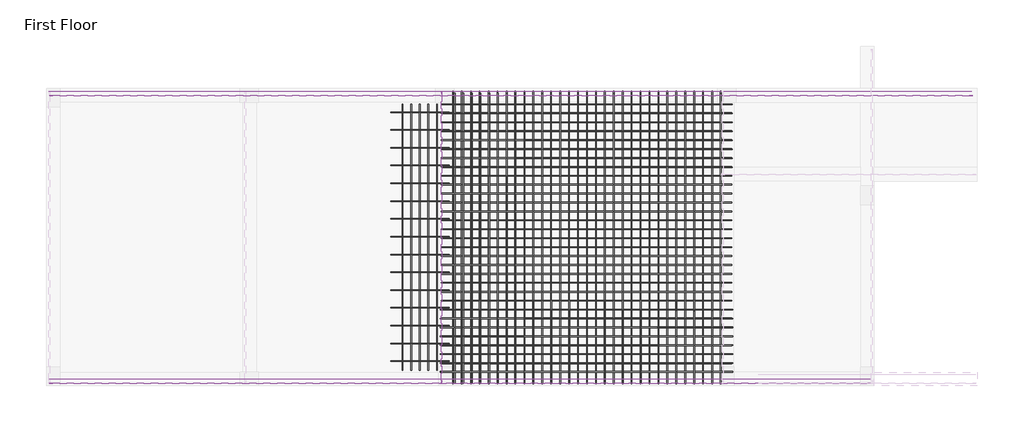
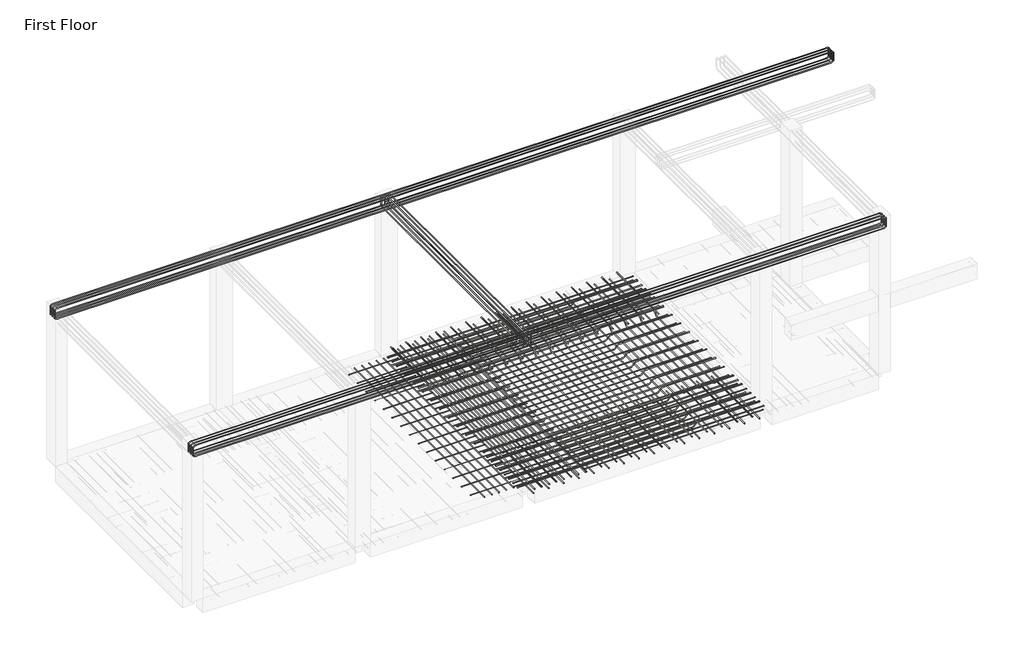
# One storey, part 3 of 4: 18 reinforcing bars.
"""IFC4 building model written with IfcOpenShell, lengths in millimetres."""

from ifc_helpers import new_model, si_unit, point, frame, origin, place, context, project, spatial, polyline, circle_curve, trimmed, segment, composite_curve, source, transform, mapped, element, save
from ifc_brep_helpers import swept_disk

model = new_model("IFC4")

# Units and contexts
model_context = context("Model", 3, world=origin())
ifc_project = project(units=[si_unit("LENGTHUNIT", "METRE", prefix="MILLI")], contexts=[model_context])

# Site, building, storey
site = spatial("IfcSite", under=ifc_project)
building = spatial("IfcBuilding", under=site)
storey = spatial("IfcBuildingStorey", under=building, Name="First Floor", Elevation=3200.4)

# Reinforcing bars
placement = place(None, origin())
reinforcing_bar_shape = source(origin(), model_context, "Body", "SolidModel", [
    swept_disk(composite_curve([segment(polyline([(-2909.6112474, 5017.2334631, 6163.6994949), (-2909.6112474, 5017.2334631, 6311.6994949)]), True, "CONTINUOUS"), segment(trimmed(circle_curve(frame((-2909.6112474, 4971.2334631, 6311.6994949), z_axis=(1.0, 0.0, 0.0), x_axis=(0.0, 46.0, 0.0)), 46.0), [point((-2909.6112474, 5017.2334631, 6311.6994949))], [point((-2909.6112474, 4971.2334631, 6357.6994949))], True, "CARTESIAN"), True, "CONTINUOUS"), segment(polyline([(-2909.6112474, 4971.2334631, 6357.6994949), (-2909.6112474, 278.4334631, 6357.6994949)]), True, "CONTINUOUS"), segment(trimmed(circle_curve(frame((-2909.6112474, 278.4334631, 6311.6994949), z_axis=(1.0, 0.0, 0.0), x_axis=(0.0, 0.0, 46.0)), 46.0), [point((-2909.6112474, 278.4334631, 6357.6994949))], [point((-2909.6112474, 232.4334631, 6311.6994949))], True, "CARTESIAN"), True, "CONTINUOUS"), segment(polyline([(-2909.6112474, 232.4334631, 6311.6994949), (-2909.6112474, 232.4334631, 6163.6994949)]), True, "CONTINUOUS")], self_intersect=False), 6.0),
])
element("IfcReinforcingBar", 1, at=placement, inside=storey, context=model_context, shape_type="MappedRepresentation", body=[
    mapped(reinforcing_bar_shape, transform((0.0, 0.0, 0.0), x_axis=(1.0, 0.0, 0.0), y_axis=(0.0, 1.0, 0.0), z_axis=(0.0, 0.0, 1.0))),
    mapped(reinforcing_bar_shape, transform((71.1994949, 0.0, 0.0), x_axis=(1.0, 0.0, 0.0), y_axis=(0.0, 1.0, 0.0), z_axis=(0.0, 0.0, 1.0))),
    mapped(reinforcing_bar_shape, transform((142.3989899, 0.0, 0.0), x_axis=(1.0, 0.0, 0.0), y_axis=(0.0, 1.0, 0.0), z_axis=(0.0, 0.0, 1.0))),
])
reinforcing_bar_2_shape = source(origin(), model_context, "Body", "SolidModel", [
    swept_disk(composite_curve([segment(polyline([(-2909.6112474, 5017.2334631, 6333.1005051), (-2909.6112474, 5017.2334631, 6185.1005051)]), True, "CONTINUOUS"), segment(trimmed(circle_curve(frame((-2909.6112474, 4971.2334631, 6185.1005051), z_axis=(-1.0, 0.0, 0.0), x_axis=(0.0, 46.0, 0.0)), 46.0), [point((-2909.6112474, 5017.2334631, 6185.1005051))], [point((-2909.6112474, 4971.2334631, 6139.1005051))], True, "CARTESIAN"), True, "CONTINUOUS"), segment(polyline([(-2909.6112474, 4971.2334631, 6139.1005051), (-2909.6112474, 278.4334631, 6139.1005051)]), True, "CONTINUOUS"), segment(trimmed(circle_curve(frame((-2909.6112474, 278.4334631, 6185.1005051), z_axis=(-1.0, 0.0, 0.0), x_axis=(0.0, 0.0, -46.0)), 46.0), [point((-2909.6112474, 278.4334631, 6139.1005051))], [point((-2909.6112474, 232.4334631, 6185.1005051))], True, "CARTESIAN"), True, "CONTINUOUS"), segment(polyline([(-2909.6112474, 232.4334631, 6185.1005051), (-2909.6112474, 232.4334631, 6333.1005051)]), True, "CONTINUOUS")], self_intersect=False), 6.0),
])
element("IfcReinforcingBar", 2, at=placement, inside=storey, context=model_context, shape_type="MappedRepresentation", body=[
    mapped(reinforcing_bar_2_shape, transform((0.0, 0.0, 0.0), x_axis=(1.0, 0.0, 0.0), y_axis=(0.0, 1.0, 0.0), z_axis=(0.0, 0.0, 1.0))),
    mapped(reinforcing_bar_2_shape, transform((71.1994949, 0.0, 0.0), x_axis=(1.0, 0.0, 0.0), y_axis=(0.0, 1.0, 0.0), z_axis=(0.0, 0.0, 1.0))),
    mapped(reinforcing_bar_2_shape, transform((142.3989899, 0.0, 0.0), x_axis=(1.0, 0.0, 0.0), y_axis=(0.0, 1.0, 0.0), z_axis=(0.0, 0.0, 1.0))),
])
reinforcing_bar_3_shape = source(origin(), model_context, "Body", "SolidModel", [
    swept_disk(composite_curve([segment(polyline([(-9325.7296265, 229.5339681, 6163.6994949), (-9325.7296265, 229.5339681, 6311.6994949)]), True, "CONTINUOUS"), segment(trimmed(circle_curve(frame((-9279.7296265, 229.5339681, 6311.6994949), z_axis=(0.0, 1.0, 0.0), x_axis=(-46.0, 0.0, 0.0)), 46.0), [point((-9325.7296265, 229.5339681, 6311.6994949))], [point((-9279.7296265, 229.5339681, 6357.6994949))], True, "CARTESIAN"), True, "CONTINUOUS"), segment(polyline([(-9279.7296265, 229.5339681, 6357.6994949), (4070.8650323, 229.5339681, 6357.6994949)]), True, "CONTINUOUS"), segment(trimmed(circle_curve(frame((4070.8650323, 229.5339681, 6311.6994949), z_axis=(0.0, 1.0, 0.0), x_axis=(0.0, 0.0, 46.0)), 46.0), [point((4070.8650323, 229.5339681, 6357.6994949))], [point((4116.8650323, 229.5339681, 6311.6994949))], True, "CARTESIAN"), True, "CONTINUOUS"), segment(polyline([(4116.8650323, 229.5339681, 6311.6994949), (4116.8650323, 229.5339681, 6163.6994949)]), True, "CONTINUOUS")], self_intersect=False), 6.0),
])
element("IfcReinforcingBar", 3, at=placement, inside=storey, context=model_context, shape_type="MappedRepresentation", body=[
    mapped(reinforcing_bar_3_shape, transform((0.0, 0.0, 0.0), x_axis=(1.0, 0.0, 0.0), y_axis=(0.0, 1.0, 0.0), z_axis=(0.0, 0.0, 1.0))),
    mapped(reinforcing_bar_3_shape, transform((0.0, 71.1994949, 0.0), x_axis=(1.0, 0.0, 0.0), y_axis=(0.0, 1.0, 0.0), z_axis=(0.0, 0.0, 1.0))),
    mapped(reinforcing_bar_3_shape, transform((0.0, 142.3989899, 0.0), x_axis=(1.0, 0.0, 0.0), y_axis=(0.0, 1.0, 0.0), z_axis=(0.0, 0.0, 1.0))),
])
reinforcing_bar_4_shape = source(origin(), model_context, "Body", "SolidModel", [
    swept_disk(composite_curve([segment(polyline([(-9326.1203644, 229.5339681, 6333.1005051), (-9326.1203644, 229.5339681, 6185.1005051)]), True, "CONTINUOUS"), segment(trimmed(circle_curve(frame((-9280.1203644, 229.5339681, 6185.1005051), z_axis=(0.0, -1.0, 0.0), x_axis=(-46.0, 0.0, 0.0)), 46.0), [point((-9326.1203644, 229.5339681, 6185.1005051))], [point((-9280.1203644, 229.5339681, 6139.1005051))], True, "CARTESIAN"), True, "CONTINUOUS"), segment(polyline([(-9280.1203644, 229.5339681, 6139.1005051), (4076.5679264, 229.5339681, 6139.1005051)]), True, "CONTINUOUS"), segment(trimmed(circle_curve(frame((4076.5679264, 229.5339681, 6185.1005051), z_axis=(0.0, -1.0, 0.0), x_axis=(0.0, 0.0, -46.0)), 46.0), [point((4076.5679264, 229.5339681, 6139.1005051))], [point((4122.5679264, 229.5339681, 6185.1005051))], True, "CARTESIAN"), True, "CONTINUOUS"), segment(polyline([(4122.5679264, 229.5339681, 6185.1005051), (4122.5679264, 229.5339681, 6333.1005051)]), True, "CONTINUOUS")], self_intersect=False), 6.0),
])
element("IfcReinforcingBar", 4, at=placement, inside=storey, context=model_context, shape_type="MappedRepresentation", body=[
    mapped(reinforcing_bar_4_shape, transform((0.0, 0.0, 0.0), x_axis=(1.0, 0.0, 0.0), y_axis=(0.0, 1.0, 0.0), z_axis=(0.0, 0.0, 1.0))),
    mapped(reinforcing_bar_4_shape, transform((0.0, 71.1994949, 0.0), x_axis=(1.0, 0.0, 0.0), y_axis=(0.0, 1.0, 0.0), z_axis=(0.0, 0.0, 1.0))),
    mapped(reinforcing_bar_4_shape, transform((0.0, 142.3989899, 0.0), x_axis=(1.0, 0.0, 0.0), y_axis=(0.0, 1.0, 0.0), z_axis=(0.0, 0.0, 1.0))),
])
reinforcing_bar_5_shape = source(origin(), model_context, "Body", "SolidModel", [
    swept_disk(composite_curve([segment(polyline([(-9325.7296265, 4879.1314555, 6162.3020076), (-9325.7296265, 4879.1314555, 6310.3020076)]), True, "CONTINUOUS"), segment(trimmed(circle_curve(frame((-9279.7296265, 4879.1314555, 6310.3020076), z_axis=(0.0, 1.0, 0.0), x_axis=(-46.0, 0.0, 0.0)), 46.0), [point((-9325.7296265, 4879.1314555, 6310.3020076))], [point((-9279.7296265, 4879.1314555, 6356.3020076))], True, "CARTESIAN"), True, "CONTINUOUS"), segment(polyline([(-9279.7296265, 4879.1314555, 6356.3020076), (5739.4882476, 4879.1314555, 6356.3020076)]), True, "CONTINUOUS"), segment(trimmed(circle_curve(frame((5739.4882476, 4879.1314555, 6310.3020076), z_axis=(0.0, 1.0, 0.0), x_axis=(0.0, 0.0, 46.0)), 46.0), [point((5739.4882476, 4879.1314555, 6356.3020076))], [point((5785.4882476, 4879.1314555, 6310.3020076))], True, "CARTESIAN"), True, "CONTINUOUS"), segment(polyline([(5785.4882476, 4879.1314555, 6310.3020076), (5785.4882476, 4879.1314555, 6162.3020076)]), True, "CONTINUOUS")], self_intersect=False), 6.0),
])
element("IfcReinforcingBar", 5, at=placement, inside=storey, context=model_context, shape_type="MappedRepresentation", body=[
    mapped(reinforcing_bar_5_shape, transform((0.0, 0.0, 0.0), x_axis=(1.0, 0.0, 0.0), y_axis=(0.0, 1.0, 0.0), z_axis=(0.0, 0.0, 1.0))),
    mapped(reinforcing_bar_5_shape, transform((0.0, 69.8020076, 0.0), x_axis=(1.0, 0.0, 0.0), y_axis=(0.0, 1.0, 0.0), z_axis=(0.0, 0.0, 1.0))),
    mapped(reinforcing_bar_5_shape, transform((0.0, 139.6040151, 0.0), x_axis=(1.0, 0.0, 0.0), y_axis=(0.0, 1.0, 0.0), z_axis=(0.0, 0.0, 1.0))),
])
reinforcing_bar_6_shape = source(origin(), model_context, "Body", "SolidModel", [
    swept_disk(composite_curve([segment(polyline([(-9326.1203644, 4879.1314555, 6334.8479924), (-9326.1203644, 4879.1314555, 6186.8479924)]), True, "CONTINUOUS"), segment(trimmed(circle_curve(frame((-9280.1203644, 4879.1314555, 6186.8479924), z_axis=(0.0, -1.0, 0.0), x_axis=(-46.0, 0.0, 0.0)), 46.0), [point((-9326.1203644, 4879.1314555, 6186.8479924))], [point((-9280.1203644, 4879.1314555, 6140.8479924))], True, "CARTESIAN"), True, "CONTINUOUS"), segment(polyline([(-9280.1203644, 4879.1314555, 6140.8479924), (5727.8951301, 4879.1314555, 6140.8479924)]), True, "CONTINUOUS"), segment(trimmed(circle_curve(frame((5727.8951301, 4879.1314555, 6186.8479924), z_axis=(0.0, -1.0, 0.0), x_axis=(0.0, 0.0, -46.0)), 46.0), [point((5727.8951301, 4879.1314555, 6140.8479924))], [point((5773.8951301, 4879.1314555, 6186.8479924))], True, "CARTESIAN"), True, "CONTINUOUS"), segment(polyline([(5773.8951301, 4879.1314555, 6186.8479924), (5773.8951301, 4879.1314555, 6334.8479924)]), True, "CONTINUOUS")], self_intersect=False), 6.0),
])
element("IfcReinforcingBar", 6, at=placement, inside=storey, context=model_context, shape_type="MappedRepresentation", body=[
    mapped(reinforcing_bar_6_shape, transform((0.0, 0.0, 0.0), x_axis=(1.0, 0.0, 0.0), y_axis=(0.0, 1.0, 0.0), z_axis=(0.0, 0.0, 1.0))),
    mapped(reinforcing_bar_6_shape, transform((0.0, 69.8020076, 0.0), x_axis=(1.0, 0.0, 0.0), y_axis=(0.0, 1.0, 0.0), z_axis=(0.0, 0.0, 1.0))),
    mapped(reinforcing_bar_6_shape, transform((0.0, 139.6040151, 0.0), x_axis=(1.0, 0.0, 0.0), y_axis=(0.0, 1.0, 0.0), z_axis=(0.0, 0.0, 1.0))),
])
reinforcing_bar_7_shape = source(origin(), model_context, "Body", "SolidModel", [
    swept_disk(composite_curve([segment(polyline([(-3546.4250876, 4809.6334631, 3159.1006995), (-3546.4250876, 440.0334631, 3159.1006995)]), True, "CONTINUOUS")], self_intersect=False), 6.0),
])
element("IfcReinforcingBar", 7, at=placement, inside=storey, context=model_context, shape_type="MappedRepresentation", body=[
    mapped(reinforcing_bar_7_shape, transform((0.0, 0.0, 0.0), x_axis=(1.0, 0.0, 0.0), y_axis=(0.0, 1.0, 0.0), z_axis=(0.0, 0.0, 1.0))),
    mapped(reinforcing_bar_7_shape, transform((140.6783338, 0.0, 0.0), x_axis=(1.0, 0.0, 0.0), y_axis=(0.0, 1.0, 0.0), z_axis=(0.0, 0.0, 1.0))),
    mapped(reinforcing_bar_7_shape, transform((281.3566676, 0.0, 0.0), x_axis=(1.0, 0.0, 0.0), y_axis=(0.0, 1.0, 0.0), z_axis=(0.0, 0.0, 1.0))),
    mapped(reinforcing_bar_7_shape, transform((422.0350014, 0.0, 0.0), x_axis=(1.0, 0.0, 0.0), y_axis=(0.0, 1.0, 0.0), z_axis=(0.0, 0.0, 1.0))),
    mapped(reinforcing_bar_7_shape, transform((562.7133352, 0.0, 0.0), x_axis=(1.0, 0.0, 0.0), y_axis=(0.0, 1.0, 0.0), z_axis=(0.0, 0.0, 1.0))),
])
reinforcing_bar_8_shape = source(origin(), model_context, "Body", "SolidModel", [
    swept_disk(composite_curve([segment(polyline([(-2778.2123639, 4678.4115375, 3171.4), (-3737.2865297, 4678.4115375, 3171.4)]), True, "CONTINUOUS")], self_intersect=False), 4.0),
])
element("IfcReinforcingBar", 8, at=placement, inside=storey, context=model_context, shape_type="MappedRepresentation", body=[
    mapped(reinforcing_bar_8_shape, transform((0.0, 0.0, 0.0), x_axis=(1.0, 0.0, 0.0), y_axis=(0.0, 1.0, 0.0), z_axis=(0.0, 0.0, 1.0))),
    mapped(reinforcing_bar_8_shape, transform((0.0, -291.8025106, 0.0), x_axis=(1.0, 0.0, 0.0), y_axis=(0.0, 1.0, 0.0), z_axis=(0.0, 0.0, 1.0))),
    mapped(reinforcing_bar_8_shape, transform((0.0, -583.6050212, 0.0), x_axis=(1.0, 0.0, 0.0), y_axis=(0.0, 1.0, 0.0), z_axis=(0.0, 0.0, 1.0))),
    mapped(reinforcing_bar_8_shape, transform((0.0, -875.4075319, 0.0), x_axis=(1.0, 0.0, 0.0), y_axis=(0.0, 1.0, 0.0), z_axis=(0.0, 0.0, 1.0))),
    mapped(reinforcing_bar_8_shape, transform((0.0, -1167.2100425, 0.0), x_axis=(1.0, 0.0, 0.0), y_axis=(0.0, 1.0, 0.0), z_axis=(0.0, 0.0, 1.0))),
    mapped(reinforcing_bar_8_shape, transform((0.0, -1459.0125531, 0.0), x_axis=(1.0, 0.0, 0.0), y_axis=(0.0, 1.0, 0.0), z_axis=(0.0, 0.0, 1.0))),
    mapped(reinforcing_bar_8_shape, transform((0.0, -1750.8150637, 0.0), x_axis=(1.0, 0.0, 0.0), y_axis=(0.0, 1.0, 0.0), z_axis=(0.0, 0.0, 1.0))),
    mapped(reinforcing_bar_8_shape, transform((0.0, -2042.6175743, 0.0), x_axis=(1.0, 0.0, 0.0), y_axis=(0.0, 1.0, 0.0), z_axis=(0.0, 0.0, 1.0))),
    mapped(reinforcing_bar_8_shape, transform((0.0, -2334.420085, 0.0), x_axis=(1.0, 0.0, 0.0), y_axis=(0.0, 1.0, 0.0), z_axis=(0.0, 0.0, 1.0))),
    mapped(reinforcing_bar_8_shape, transform((0.0, -2626.2225956, 0.0), x_axis=(1.0, 0.0, 0.0), y_axis=(0.0, 1.0, 0.0), z_axis=(0.0, 0.0, 1.0))),
    mapped(reinforcing_bar_8_shape, transform((0.0, -2918.0251062, 0.0), x_axis=(1.0, 0.0, 0.0), y_axis=(0.0, 1.0, 0.0), z_axis=(0.0, 0.0, 1.0))),
    mapped(reinforcing_bar_8_shape, transform((0.0, -3209.8276168, 0.0), x_axis=(1.0, 0.0, 0.0), y_axis=(0.0, 1.0, 0.0), z_axis=(0.0, 0.0, 1.0))),
    mapped(reinforcing_bar_8_shape, transform((0.0, -3501.6301274, 0.0), x_axis=(1.0, 0.0, 0.0), y_axis=(0.0, 1.0, 0.0), z_axis=(0.0, 0.0, 1.0))),
    mapped(reinforcing_bar_8_shape, transform((0.0, -3793.4326381, 0.0), x_axis=(1.0, 0.0, 0.0), y_axis=(0.0, 1.0, 0.0), z_axis=(0.0, 0.0, 1.0))),
    mapped(reinforcing_bar_8_shape, transform((0.0, -4085.2351487, 0.0), x_axis=(1.0, 0.0, 0.0), y_axis=(0.0, 1.0, 0.0), z_axis=(0.0, 0.0, 1.0))),
])
reinforcing_bar_9_shape = source(origin(), model_context, "Body", "SolidModel", [
    swept_disk(composite_curve([segment(polyline([(-1702.6950858, 4992.3164819, 3154.1006995), (-1702.6950858, 234.3272052, 3154.1006995)]), True, "CONTINUOUS")], self_intersect=False), 6.0),
])
element("IfcReinforcingBar", 9, at=placement, inside=storey, context=model_context, shape_type="MappedRepresentation", body=[
    mapped(reinforcing_bar_9_shape, transform((0.0, 0.0, 0.0), x_axis=(1.0, 0.0, 0.0), y_axis=(0.0, 1.0, 0.0), z_axis=(0.0, 0.0, 1.0))),
    mapped(reinforcing_bar_9_shape, transform((-141.4880952, 0.0, 0.0), x_axis=(1.0, 0.0, 0.0), y_axis=(0.0, 1.0, 0.0), z_axis=(0.0, 0.0, 1.0))),
    mapped(reinforcing_bar_9_shape, transform((-282.9761905, 0.0, 0.0), x_axis=(1.0, 0.0, 0.0), y_axis=(0.0, 1.0, 0.0), z_axis=(0.0, 0.0, 1.0))),
    mapped(reinforcing_bar_9_shape, transform((-424.4642857, 0.0, 0.0), x_axis=(1.0, 0.0, 0.0), y_axis=(0.0, 1.0, 0.0), z_axis=(0.0, 0.0, 1.0))),
    mapped(reinforcing_bar_9_shape, transform((-565.952381, 0.0, 0.0), x_axis=(1.0, 0.0, 0.0), y_axis=(0.0, 1.0, 0.0), z_axis=(0.0, 0.0, 1.0))),
    mapped(reinforcing_bar_9_shape, transform((-707.4404762, 0.0, 0.0), x_axis=(1.0, 0.0, 0.0), y_axis=(0.0, 1.0, 0.0), z_axis=(0.0, 0.0, 1.0))),
    mapped(reinforcing_bar_9_shape, transform((-848.9285714, 0.0, 0.0), x_axis=(1.0, 0.0, 0.0), y_axis=(0.0, 1.0, 0.0), z_axis=(0.0, 0.0, 1.0))),
    mapped(reinforcing_bar_9_shape, transform((-990.4166667, 0.0, 0.0), x_axis=(1.0, 0.0, 0.0), y_axis=(0.0, 1.0, 0.0), z_axis=(0.0, 0.0, 1.0))),
])
reinforcing_bar_10_shape = source(origin(), model_context, "Body", "SolidModel", [
    swept_disk(composite_curve([segment(polyline([(-2905.905155, 4803.6334631, 3166.3687876), (-1727.9771661, 4803.6334631, 3166.3687876)]), True, "CONTINUOUS"), segment(trimmed(circle_curve(frame((-1727.9771661, 4803.6334631, 3120.3687876), z_axis=(0.0, 1.0, 0.0), x_axis=(0.0, 0.0, 46.0)), 46.0), [point((-1727.9771661, 4803.6334631, 3166.3687876))], [point((-1695.4502541, 4803.6334631, 3152.8956996))], True, "CARTESIAN"), True, "CONTINUOUS"), segment(polyline([(-1695.4502541, 4803.6334631, 3152.8956996), (-1634.9899166, 4803.6334631, 3092.4353621)]), True, "CONTINUOUS"), segment(trimmed(circle_curve(frame((-1602.4630047, 4803.6334631, 3124.962274), z_axis=(0.0, -1.0, 0.0), x_axis=(-32.52691189999996, 0.0, -32.52691189999996)), 46.0), [point((-1634.9899166, 4803.6334631, 3092.4353621))], [point((-1602.4630047, 4803.6334631, 3078.962274))], True, "CARTESIAN"), True, "CONTINUOUS"), segment(polyline([(-1602.4630047, 4803.6334631, 3078.962274), (1847.5013288, 4803.6334631, 3078.962274)]), True, "CONTINUOUS")], self_intersect=False), 6.0),
])
element("IfcReinforcingBar", 10, at=placement, inside=storey, context=model_context, shape_type="MappedRepresentation", body=[
    mapped(reinforcing_bar_10_shape, transform((0.0, 0.0, 0.0), x_axis=(1.0, 0.0, 0.0), y_axis=(0.0, 1.0, 0.0), z_axis=(0.0, 0.0, 1.0))),
    mapped(reinforcing_bar_10_shape, transform((0.0, -292.3066667, 0.0), x_axis=(1.0, 0.0, 0.0), y_axis=(0.0, 1.0, 0.0), z_axis=(0.0, 0.0, 1.0))),
    mapped(reinforcing_bar_10_shape, transform((0.0, -584.6133333, 0.0), x_axis=(1.0, 0.0, 0.0), y_axis=(0.0, 1.0, 0.0), z_axis=(0.0, 0.0, 1.0))),
    mapped(reinforcing_bar_10_shape, transform((0.0, -876.92, 0.0), x_axis=(1.0, 0.0, 0.0), y_axis=(0.0, 1.0, 0.0), z_axis=(0.0, 0.0, 1.0))),
    mapped(reinforcing_bar_10_shape, transform((0.0, -1169.2266667, 0.0), x_axis=(1.0, 0.0, 0.0), y_axis=(0.0, 1.0, 0.0), z_axis=(0.0, 0.0, 1.0))),
    mapped(reinforcing_bar_10_shape, transform((0.0, -1461.5333333, 0.0), x_axis=(1.0, 0.0, 0.0), y_axis=(0.0, 1.0, 0.0), z_axis=(0.0, 0.0, 1.0))),
    mapped(reinforcing_bar_10_shape, transform((0.0, -1753.84, 0.0), x_axis=(1.0, 0.0, 0.0), y_axis=(0.0, 1.0, 0.0), z_axis=(0.0, 0.0, 1.0))),
    mapped(reinforcing_bar_10_shape, transform((0.0, -2046.1466667, 0.0), x_axis=(1.0, 0.0, 0.0), y_axis=(0.0, 1.0, 0.0), z_axis=(0.0, 0.0, 1.0))),
    mapped(reinforcing_bar_10_shape, transform((0.0, -2338.4533333, 0.0), x_axis=(1.0, 0.0, 0.0), y_axis=(0.0, 1.0, 0.0), z_axis=(0.0, 0.0, 1.0))),
    mapped(reinforcing_bar_10_shape, transform((0.0, -2630.76, 0.0), x_axis=(1.0, 0.0, 0.0), y_axis=(0.0, 1.0, 0.0), z_axis=(0.0, 0.0, 1.0))),
    mapped(reinforcing_bar_10_shape, transform((0.0, -2923.0666667, 0.0), x_axis=(1.0, 0.0, 0.0), y_axis=(0.0, 1.0, 0.0), z_axis=(0.0, 0.0, 1.0))),
    mapped(reinforcing_bar_10_shape, transform((0.0, -3215.3733333, 0.0), x_axis=(1.0, 0.0, 0.0), y_axis=(0.0, 1.0, 0.0), z_axis=(0.0, 0.0, 1.0))),
    mapped(reinforcing_bar_10_shape, transform((0.0, -3507.68, 0.0), x_axis=(1.0, 0.0, 0.0), y_axis=(0.0, 1.0, 0.0), z_axis=(0.0, 0.0, 1.0))),
    mapped(reinforcing_bar_10_shape, transform((0.0, -3799.9866667, 0.0), x_axis=(1.0, 0.0, 0.0), y_axis=(0.0, 1.0, 0.0), z_axis=(0.0, 0.0, 1.0))),
    mapped(reinforcing_bar_10_shape, transform((0.0, -4092.2933333, 0.0), x_axis=(1.0, 0.0, 0.0), y_axis=(0.0, 1.0, 0.0), z_axis=(0.0, 0.0, 1.0))),
    mapped(reinforcing_bar_10_shape, transform((0.0, -4384.6, 0.0), x_axis=(1.0, 0.0, 0.0), y_axis=(0.0, 1.0, 0.0), z_axis=(0.0, 0.0, 1.0))),
])
reinforcing_bar_11_shape = source(origin(), model_context, "Body", "SolidModel", [
    swept_disk(composite_curve([segment(polyline([(-2911.6309684, 4803.6334631, 3163.8017937), (-1557.9199073, 4803.6334631, 3163.8017937)]), True, "CONTINUOUS")], self_intersect=False), 6.0),
])
element("IfcReinforcingBar", 11, at=placement, inside=storey, context=model_context, shape_type="MappedRepresentation", body=[
    mapped(reinforcing_bar_11_shape, transform((0.0, 0.0, 0.0), x_axis=(1.0, 0.0, 0.0), y_axis=(0.0, 1.0, 0.0), z_axis=(0.0, 0.0, 1.0))),
    mapped(reinforcing_bar_11_shape, transform((0.0, -292.3066667, 0.0), x_axis=(1.0, 0.0, 0.0), y_axis=(0.0, 1.0, 0.0), z_axis=(0.0, 0.0, 1.0))),
    mapped(reinforcing_bar_11_shape, transform((0.0, -584.6133333, 0.0), x_axis=(1.0, 0.0, 0.0), y_axis=(0.0, 1.0, 0.0), z_axis=(0.0, 0.0, 1.0))),
    mapped(reinforcing_bar_11_shape, transform((0.0, -876.92, 0.0), x_axis=(1.0, 0.0, 0.0), y_axis=(0.0, 1.0, 0.0), z_axis=(0.0, 0.0, 1.0))),
    mapped(reinforcing_bar_11_shape, transform((0.0, -1169.2266667, 0.0), x_axis=(1.0, 0.0, 0.0), y_axis=(0.0, 1.0, 0.0), z_axis=(0.0, 0.0, 1.0))),
    mapped(reinforcing_bar_11_shape, transform((0.0, -1461.5333333, 0.0), x_axis=(1.0, 0.0, 0.0), y_axis=(0.0, 1.0, 0.0), z_axis=(0.0, 0.0, 1.0))),
    mapped(reinforcing_bar_11_shape, transform((0.0, -1753.84, 0.0), x_axis=(1.0, 0.0, 0.0), y_axis=(0.0, 1.0, 0.0), z_axis=(0.0, 0.0, 1.0))),
    mapped(reinforcing_bar_11_shape, transform((0.0, -2046.1466667, 0.0), x_axis=(1.0, 0.0, 0.0), y_axis=(0.0, 1.0, 0.0), z_axis=(0.0, 0.0, 1.0))),
    mapped(reinforcing_bar_11_shape, transform((0.0, -2338.4533333, 0.0), x_axis=(1.0, 0.0, 0.0), y_axis=(0.0, 1.0, 0.0), z_axis=(0.0, 0.0, 1.0))),
    mapped(reinforcing_bar_11_shape, transform((0.0, -2630.76, 0.0), x_axis=(1.0, 0.0, 0.0), y_axis=(0.0, 1.0, 0.0), z_axis=(0.0, 0.0, 1.0))),
    mapped(reinforcing_bar_11_shape, transform((0.0, -2923.0666667, 0.0), x_axis=(1.0, 0.0, 0.0), y_axis=(0.0, 1.0, 0.0), z_axis=(0.0, 0.0, 1.0))),
    mapped(reinforcing_bar_11_shape, transform((0.0, -3215.3733333, 0.0), x_axis=(1.0, 0.0, 0.0), y_axis=(0.0, 1.0, 0.0), z_axis=(0.0, 0.0, 1.0))),
    mapped(reinforcing_bar_11_shape, transform((0.0, -3507.68, 0.0), x_axis=(1.0, 0.0, 0.0), y_axis=(0.0, 1.0, 0.0), z_axis=(0.0, 0.0, 1.0))),
    mapped(reinforcing_bar_11_shape, transform((0.0, -3799.9866667, 0.0), x_axis=(1.0, 0.0, 0.0), y_axis=(0.0, 1.0, 0.0), z_axis=(0.0, 0.0, 1.0))),
    mapped(reinforcing_bar_11_shape, transform((0.0, -4092.2933333, 0.0), x_axis=(1.0, 0.0, 0.0), y_axis=(0.0, 1.0, 0.0), z_axis=(0.0, 0.0, 1.0))),
    mapped(reinforcing_bar_11_shape, transform((0.0, -4384.6, 0.0), x_axis=(1.0, 0.0, 0.0), y_axis=(0.0, 1.0, 0.0), z_axis=(0.0, 0.0, 1.0))),
])
reinforcing_bar_12_shape = source(origin(), model_context, "Body", "SolidModel", [
    swept_disk(composite_curve([segment(polyline([(1849.122149, 559.2793552, 3166.3687876), (670.8521547, 559.2793552, 3166.3687876)]), True, "CONTINUOUS"), segment(trimmed(circle_curve(frame((670.8521547, 559.2793552, 3120.3687876), z_axis=(0.0, -1.0, 0.0), x_axis=(0.0, 0.0, 46.0)), 46.0), [point((670.8521547, 559.2793552, 3166.3687876))], [point((638.3252427, 559.2793552, 3152.8956996))], True, "CARTESIAN"), True, "CONTINUOUS"), segment(polyline([(638.3252427, 559.2793552, 3152.8956996), (577.8649052, 559.2793552, 3092.4353621)]), True, "CONTINUOUS"), segment(trimmed(circle_curve(frame((545.3379933, 559.2793552, 3124.962274), z_axis=(0.0, 1.0000000000000002, 0.0), x_axis=(32.52691189999996, 0.0, -32.52691189999996)), 46.0), [point((577.8649052, 559.2793552, 3092.4353621))], [point((545.3379933, 559.2793552, 3078.962274))], True, "CARTESIAN"), True, "CONTINUOUS"), segment(polyline([(545.3379933, 559.2793552, 3078.962274), (-2914.2248337, 559.2793552, 3078.962274)]), True, "CONTINUOUS")], self_intersect=False), 6.0),
])
element("IfcReinforcingBar", 12, at=placement, inside=storey, context=model_context, shape_type="MappedRepresentation", body=[
    mapped(reinforcing_bar_12_shape, transform((0.0, 0.0, 0.0), x_axis=(1.0, 0.0, 0.0), y_axis=(0.0, 1.0, 0.0), z_axis=(0.0, 0.0, 1.0))),
    mapped(reinforcing_bar_12_shape, transform((0.0, 293.1320516, 0.0), x_axis=(1.0, 0.0, 0.0), y_axis=(0.0, 1.0, 0.0), z_axis=(0.0, 0.0, 1.0))),
    mapped(reinforcing_bar_12_shape, transform((0.0, 586.2641031, 0.0), x_axis=(1.0, 0.0, 0.0), y_axis=(0.0, 1.0, 0.0), z_axis=(0.0, 0.0, 1.0))),
    mapped(reinforcing_bar_12_shape, transform((0.0, 879.3961547, 0.0), x_axis=(1.0, 0.0, 0.0), y_axis=(0.0, 1.0, 0.0), z_axis=(0.0, 0.0, 1.0))),
    mapped(reinforcing_bar_12_shape, transform((0.0, 1172.5282063, 0.0), x_axis=(1.0, 0.0, 0.0), y_axis=(0.0, 1.0, 0.0), z_axis=(0.0, 0.0, 1.0))),
    mapped(reinforcing_bar_12_shape, transform((0.0, 1465.6602578, 0.0), x_axis=(1.0, 0.0, 0.0), y_axis=(0.0, 1.0, 0.0), z_axis=(0.0, 0.0, 1.0))),
    mapped(reinforcing_bar_12_shape, transform((0.0, 1758.7923094, 0.0), x_axis=(1.0, 0.0, 0.0), y_axis=(0.0, 1.0, 0.0), z_axis=(0.0, 0.0, 1.0))),
    mapped(reinforcing_bar_12_shape, transform((0.0, 2051.924361, 0.0), x_axis=(1.0, 0.0, 0.0), y_axis=(0.0, 1.0, 0.0), z_axis=(0.0, 0.0, 1.0))),
    mapped(reinforcing_bar_12_shape, transform((0.0, 2345.0564125, 0.0), x_axis=(1.0, 0.0, 0.0), y_axis=(0.0, 1.0, 0.0), z_axis=(0.0, 0.0, 1.0))),
    mapped(reinforcing_bar_12_shape, transform((0.0, 2638.1884641, 0.0), x_axis=(1.0, 0.0, 0.0), y_axis=(0.0, 1.0, 0.0), z_axis=(0.0, 0.0, 1.0))),
    mapped(reinforcing_bar_12_shape, transform((0.0, 2931.3205157, 0.0), x_axis=(1.0, 0.0, 0.0), y_axis=(0.0, 1.0, 0.0), z_axis=(0.0, 0.0, 1.0))),
    mapped(reinforcing_bar_12_shape, transform((0.0, 3224.4525672, 0.0), x_axis=(1.0, 0.0, 0.0), y_axis=(0.0, 1.0, 0.0), z_axis=(0.0, 0.0, 1.0))),
    mapped(reinforcing_bar_12_shape, transform((0.0, 3517.5846188, 0.0), x_axis=(1.0, 0.0, 0.0), y_axis=(0.0, 1.0, 0.0), z_axis=(0.0, 0.0, 1.0))),
    mapped(reinforcing_bar_12_shape, transform((0.0, 3810.7166704, 0.0), x_axis=(1.0, 0.0, 0.0), y_axis=(0.0, 1.0, 0.0), z_axis=(0.0, 0.0, 1.0))),
    mapped(reinforcing_bar_12_shape, transform((0.0, 4103.848722, 0.0), x_axis=(1.0, 0.0, 0.0), y_axis=(0.0, 1.0, 0.0), z_axis=(0.0, 0.0, 1.0))),
])
reinforcing_bar_13_shape = source(origin(), model_context, "Body", "SolidModel", [
    swept_disk(composite_curve([segment(polyline([(1854.5084921, 3775.4003908, 3154.1006995), (-2903.4807845, 3775.4003908, 3154.1006995)]), True, "CONTINUOUS")], self_intersect=False), 6.0),
])
element("IfcReinforcingBar", 13, at=placement, inside=storey, context=model_context, shape_type="MappedRepresentation", body=[
    mapped(reinforcing_bar_13_shape, transform((0.0, 0.0, 0.0), x_axis=(1.0, 0.0, 0.0), y_axis=(0.0, 1.0, 0.0), z_axis=(0.0, 0.0, 1.0))),
    mapped(reinforcing_bar_13_shape, transform((0.0, 146.8904389, 0.0), x_axis=(1.0, 0.0, 0.0), y_axis=(0.0, 1.0, 0.0), z_axis=(0.0, 0.0, 1.0))),
    mapped(reinforcing_bar_13_shape, transform((0.0, 293.7808778, 0.0), x_axis=(1.0, 0.0, 0.0), y_axis=(0.0, 1.0, 0.0), z_axis=(0.0, 0.0, 1.0))),
    mapped(reinforcing_bar_13_shape, transform((0.0, 440.6713167, 0.0), x_axis=(1.0, 0.0, 0.0), y_axis=(0.0, 1.0, 0.0), z_axis=(0.0, 0.0, 1.0))),
    mapped(reinforcing_bar_13_shape, transform((0.0, 587.5617556, 0.0), x_axis=(1.0, 0.0, 0.0), y_axis=(0.0, 1.0, 0.0), z_axis=(0.0, 0.0, 1.0))),
    mapped(reinforcing_bar_13_shape, transform((0.0, 734.4521945, 0.0), x_axis=(1.0, 0.0, 0.0), y_axis=(0.0, 1.0, 0.0), z_axis=(0.0, 0.0, 1.0))),
    mapped(reinforcing_bar_13_shape, transform((0.0, 881.3426334, 0.0), x_axis=(1.0, 0.0, 0.0), y_axis=(0.0, 1.0, 0.0), z_axis=(0.0, 0.0, 1.0))),
    mapped(reinforcing_bar_13_shape, transform((0.0, 1028.2330723, 0.0), x_axis=(1.0, 0.0, 0.0), y_axis=(0.0, 1.0, 0.0), z_axis=(0.0, 0.0, 1.0))),
])
reinforcing_bar_14_shape = source(origin(), model_context, "Body", "SolidModel", [
    swept_disk(composite_curve([segment(polyline([(1667.8254733, 4978.61046, 3166.3687876), (1667.8254733, 3800.6824711, 3166.3687876)]), True, "CONTINUOUS"), segment(trimmed(circle_curve(frame((1667.8254733, 3800.6824711, 3120.3687876), z_axis=(1.0, 0.0, 0.0), x_axis=(0.0, 0.0, 46.0)), 46.0), [point((1667.8254733, 3800.6824711, 3166.3687876))], [point((1667.8254733, 3768.1555592, 3152.8956996))], True, "CARTESIAN"), True, "CONTINUOUS"), segment(polyline([(1667.8254733, 3768.1555592, 3152.8956996), (1667.8254733, 3707.6952216, 3092.4353621)]), True, "CONTINUOUS"), segment(trimmed(circle_curve(frame((1667.8254733, 3675.1683097, 3124.962274), z_axis=(-1.0, 0.0, 0.0), x_axis=(0.0, 32.52691189999996, -32.52691189999996)), 46.0), [point((1667.8254733, 3707.6952216, 3092.4353621))], [point((1667.8254733, 3675.1683097, 3078.962274))], True, "CARTESIAN"), True, "CONTINUOUS"), segment(polyline([(1667.8254733, 3675.1683097, 3078.962274), (1667.8254733, 225.2039762, 3078.962274)]), True, "CONTINUOUS")], self_intersect=False), 6.0),
])
element("IfcReinforcingBar", 14, at=placement, inside=storey, context=model_context, shape_type="MappedRepresentation", body=[
    mapped(reinforcing_bar_14_shape, transform((0.0, 0.0, 0.0), x_axis=(1.0, 0.0, 0.0), y_axis=(0.0, 1.0, 0.0), z_axis=(0.0, 0.0, 1.0))),
    mapped(reinforcing_bar_14_shape, transform((-292.44, 0.0, 0.0), x_axis=(1.0, 0.0, 0.0), y_axis=(0.0, 1.0, 0.0), z_axis=(0.0, 0.0, 1.0))),
    mapped(reinforcing_bar_14_shape, transform((-584.88, 0.0, 0.0), x_axis=(1.0, 0.0, 0.0), y_axis=(0.0, 1.0, 0.0), z_axis=(0.0, 0.0, 1.0))),
    mapped(reinforcing_bar_14_shape, transform((-877.32, 0.0, 0.0), x_axis=(1.0, 0.0, 0.0), y_axis=(0.0, 1.0, 0.0), z_axis=(0.0, 0.0, 1.0))),
    mapped(reinforcing_bar_14_shape, transform((-1169.76, 0.0, 0.0), x_axis=(1.0, 0.0, 0.0), y_axis=(0.0, 1.0, 0.0), z_axis=(0.0, 0.0, 1.0))),
    mapped(reinforcing_bar_14_shape, transform((-1462.2, 0.0, 0.0), x_axis=(1.0, 0.0, 0.0), y_axis=(0.0, 1.0, 0.0), z_axis=(0.0, 0.0, 1.0))),
    mapped(reinforcing_bar_14_shape, transform((-1754.64, 0.0, 0.0), x_axis=(1.0, 0.0, 0.0), y_axis=(0.0, 1.0, 0.0), z_axis=(0.0, 0.0, 1.0))),
    mapped(reinforcing_bar_14_shape, transform((-2047.08, 0.0, 0.0), x_axis=(1.0, 0.0, 0.0), y_axis=(0.0, 1.0, 0.0), z_axis=(0.0, 0.0, 1.0))),
    mapped(reinforcing_bar_14_shape, transform((-2339.52, 0.0, 0.0), x_axis=(1.0, 0.0, 0.0), y_axis=(0.0, 1.0, 0.0), z_axis=(0.0, 0.0, 1.0))),
    mapped(reinforcing_bar_14_shape, transform((-2631.96, 0.0, 0.0), x_axis=(1.0, 0.0, 0.0), y_axis=(0.0, 1.0, 0.0), z_axis=(0.0, 0.0, 1.0))),
    mapped(reinforcing_bar_14_shape, transform((-2924.4, 0.0, 0.0), x_axis=(1.0, 0.0, 0.0), y_axis=(0.0, 1.0, 0.0), z_axis=(0.0, 0.0, 1.0))),
    mapped(reinforcing_bar_14_shape, transform((-3216.84, 0.0, 0.0), x_axis=(1.0, 0.0, 0.0), y_axis=(0.0, 1.0, 0.0), z_axis=(0.0, 0.0, 1.0))),
    mapped(reinforcing_bar_14_shape, transform((-3509.28, 0.0, 0.0), x_axis=(1.0, 0.0, 0.0), y_axis=(0.0, 1.0, 0.0), z_axis=(0.0, 0.0, 1.0))),
    mapped(reinforcing_bar_14_shape, transform((-3801.72, 0.0, 0.0), x_axis=(1.0, 0.0, 0.0), y_axis=(0.0, 1.0, 0.0), z_axis=(0.0, 0.0, 1.0))),
    mapped(reinforcing_bar_14_shape, transform((-4094.16, 0.0, 0.0), x_axis=(1.0, 0.0, 0.0), y_axis=(0.0, 1.0, 0.0), z_axis=(0.0, 0.0, 1.0))),
    mapped(reinforcing_bar_14_shape, transform((-4386.6, 0.0, 0.0), x_axis=(1.0, 0.0, 0.0), y_axis=(0.0, 1.0, 0.0), z_axis=(0.0, 0.0, 1.0))),
])
reinforcing_bar_15_shape = source(origin(), model_context, "Body", "SolidModel", [
    swept_disk(composite_curve([segment(polyline([(1667.8254733, 5026.3578219, 3163.8017937), (1667.8254733, 3630.6252123, 3163.8017937)]), True, "CONTINUOUS")], self_intersect=False), 6.0),
])
element("IfcReinforcingBar", 15, at=placement, inside=storey, context=model_context, shape_type="MappedRepresentation", body=[
    mapped(reinforcing_bar_15_shape, transform((0.0, 0.0, 0.0), x_axis=(1.0, 0.0, 0.0), y_axis=(0.0, 1.0, 0.0), z_axis=(0.0, 0.0, 1.0))),
    mapped(reinforcing_bar_15_shape, transform((-292.44, 0.0, 0.0), x_axis=(1.0, 0.0, 0.0), y_axis=(0.0, 1.0, 0.0), z_axis=(0.0, 0.0, 1.0))),
    mapped(reinforcing_bar_15_shape, transform((-584.88, 0.0, 0.0), x_axis=(1.0, 0.0, 0.0), y_axis=(0.0, 1.0, 0.0), z_axis=(0.0, 0.0, 1.0))),
    mapped(reinforcing_bar_15_shape, transform((-877.32, 0.0, 0.0), x_axis=(1.0, 0.0, 0.0), y_axis=(0.0, 1.0, 0.0), z_axis=(0.0, 0.0, 1.0))),
    mapped(reinforcing_bar_15_shape, transform((-1169.76, 0.0, 0.0), x_axis=(1.0, 0.0, 0.0), y_axis=(0.0, 1.0, 0.0), z_axis=(0.0, 0.0, 1.0))),
    mapped(reinforcing_bar_15_shape, transform((-1462.2, 0.0, 0.0), x_axis=(1.0, 0.0, 0.0), y_axis=(0.0, 1.0, 0.0), z_axis=(0.0, 0.0, 1.0))),
    mapped(reinforcing_bar_15_shape, transform((-1754.64, 0.0, 0.0), x_axis=(1.0, 0.0, 0.0), y_axis=(0.0, 1.0, 0.0), z_axis=(0.0, 0.0, 1.0))),
    mapped(reinforcing_bar_15_shape, transform((-2047.08, 0.0, 0.0), x_axis=(1.0, 0.0, 0.0), y_axis=(0.0, 1.0, 0.0), z_axis=(0.0, 0.0, 1.0))),
    mapped(reinforcing_bar_15_shape, transform((-2339.52, 0.0, 0.0), x_axis=(1.0, 0.0, 0.0), y_axis=(0.0, 1.0, 0.0), z_axis=(0.0, 0.0, 1.0))),
    mapped(reinforcing_bar_15_shape, transform((-2631.96, 0.0, 0.0), x_axis=(1.0, 0.0, 0.0), y_axis=(0.0, 1.0, 0.0), z_axis=(0.0, 0.0, 1.0))),
    mapped(reinforcing_bar_15_shape, transform((-2924.4, 0.0, 0.0), x_axis=(1.0, 0.0, 0.0), y_axis=(0.0, 1.0, 0.0), z_axis=(0.0, 0.0, 1.0))),
    mapped(reinforcing_bar_15_shape, transform((-3216.84, 0.0, 0.0), x_axis=(1.0, 0.0, 0.0), y_axis=(0.0, 1.0, 0.0), z_axis=(0.0, 0.0, 1.0))),
    mapped(reinforcing_bar_15_shape, transform((-3509.28, 0.0, 0.0), x_axis=(1.0, 0.0, 0.0), y_axis=(0.0, 1.0, 0.0), z_axis=(0.0, 0.0, 1.0))),
    mapped(reinforcing_bar_15_shape, transform((-3801.72, 0.0, 0.0), x_axis=(1.0, 0.0, 0.0), y_axis=(0.0, 1.0, 0.0), z_axis=(0.0, 0.0, 1.0))),
    mapped(reinforcing_bar_15_shape, transform((-4094.16, 0.0, 0.0), x_axis=(1.0, 0.0, 0.0), y_axis=(0.0, 1.0, 0.0), z_axis=(0.0, 0.0, 1.0))),
    mapped(reinforcing_bar_15_shape, transform((-4386.6, 0.0, 0.0), x_axis=(1.0, 0.0, 0.0), y_axis=(0.0, 1.0, 0.0), z_axis=(0.0, 0.0, 1.0))),
])
reinforcing_bar_16_shape = source(origin(), model_context, "Body", "SolidModel", [
    swept_disk(composite_curve([segment(polyline([(1861.271842, 1438.6755099, 3154.4697281), (-2926.3745267, 1438.6755099, 3154.4697281)]), True, "CONTINUOUS")], self_intersect=False), 6.0),
])
element("IfcReinforcingBar", 16, at=placement, inside=storey, context=model_context, shape_type="MappedRepresentation", body=[
    mapped(reinforcing_bar_16_shape, transform((0.0, 0.0, 0.0), x_axis=(1.0, 0.0, 0.0), y_axis=(0.0, 1.0, 0.0), z_axis=(0.0, 0.0, 1.0))),
    mapped(reinforcing_bar_16_shape, transform((0.0, -145.6631495, 0.0), x_axis=(1.0, 0.0, 0.0), y_axis=(0.0, 1.0, 0.0), z_axis=(0.0, 0.0, 1.0))),
    mapped(reinforcing_bar_16_shape, transform((0.0, -291.3262991, 0.0), x_axis=(1.0, 0.0, 0.0), y_axis=(0.0, 1.0, 0.0), z_axis=(0.0, 0.0, 1.0))),
    mapped(reinforcing_bar_16_shape, transform((0.0, -436.9894486, 0.0), x_axis=(1.0, 0.0, 0.0), y_axis=(0.0, 1.0, 0.0), z_axis=(0.0, 0.0, 1.0))),
    mapped(reinforcing_bar_16_shape, transform((0.0, -582.6525982, 0.0), x_axis=(1.0, 0.0, 0.0), y_axis=(0.0, 1.0, 0.0), z_axis=(0.0, 0.0, 1.0))),
    mapped(reinforcing_bar_16_shape, transform((0.0, -728.3157477, 0.0), x_axis=(1.0, 0.0, 0.0), y_axis=(0.0, 1.0, 0.0), z_axis=(0.0, 0.0, 1.0))),
    mapped(reinforcing_bar_16_shape, transform((0.0, -873.9788973, 0.0), x_axis=(1.0, 0.0, 0.0), y_axis=(0.0, 1.0, 0.0), z_axis=(0.0, 0.0, 1.0))),
    mapped(reinforcing_bar_16_shape, transform((0.0, -1019.6420468, 0.0), x_axis=(1.0, 0.0, 0.0), y_axis=(0.0, 1.0, 0.0), z_axis=(0.0, 0.0, 1.0))),
])
reinforcing_bar_17_shape = source(origin(), model_context, "Body", "SolidModel", [
    swept_disk(composite_curve([segment(polyline([(-2578.5286346, 223.5831561, 3166.3687876), (-2578.5286346, 1401.8531503, 3166.3687876)]), True, "CONTINUOUS"), segment(trimmed(circle_curve(frame((-2578.5286346, 1401.8531503, 3120.3687876), z_axis=(-1.0, 0.0, 0.0), x_axis=(0.0, 0.0, 46.0)), 46.0), [point((-2578.5286346, 1401.8531503, 3166.3687876))], [point((-2578.5286346, 1434.3800623, 3152.8956996))], True, "CARTESIAN"), True, "CONTINUOUS"), segment(polyline([(-2578.5286346, 1434.3800623, 3152.8956996), (-2578.5286346, 1494.8026738, 3092.4730881)]), True, "CONTINUOUS"), segment(trimmed(circle_curve(frame((-2578.5286346, 1527.3295857, 3125.0), z_axis=(1.0, 0.0, 0.0), x_axis=(0.0, -32.52691189999996, -32.52691189999996)), 46.0), [point((-2578.5286346, 1494.8026738, 3092.4730881))], [point((-2578.5286346, 1527.3295857, 3079.0))], True, "CARTESIAN"), True, "CONTINUOUS"), segment(polyline([(-2578.5286346, 1527.3295857, 3079.0), (-2578.5286346, 5025.6536732, 3079.0)]), True, "CONTINUOUS")], self_intersect=False), 6.0),
])
element("IfcReinforcingBar", 17, at=placement, inside=storey, context=model_context, shape_type="MappedRepresentation", body=[
    mapped(reinforcing_bar_17_shape, transform((0.0, 0.0, 0.0), x_axis=(1.0, 0.0, 0.0), y_axis=(0.0, 1.0, 0.0), z_axis=(0.0, 0.0, 1.0))),
    mapped(reinforcing_bar_17_shape, transform((293.1320516, 0.0, 0.0), x_axis=(1.0, 0.0, 0.0), y_axis=(0.0, 1.0, 0.0), z_axis=(0.0, 0.0, 1.0))),
    mapped(reinforcing_bar_17_shape, transform((586.2641031, 0.0, 0.0), x_axis=(1.0, 0.0, 0.0), y_axis=(0.0, 1.0, 0.0), z_axis=(0.0, 0.0, 1.0))),
    mapped(reinforcing_bar_17_shape, transform((879.3961547, 0.0, 0.0), x_axis=(1.0, 0.0, 0.0), y_axis=(0.0, 1.0, 0.0), z_axis=(0.0, 0.0, 1.0))),
    mapped(reinforcing_bar_17_shape, transform((1172.5282063, 0.0, 0.0), x_axis=(1.0, 0.0, 0.0), y_axis=(0.0, 1.0, 0.0), z_axis=(0.0, 0.0, 1.0))),
    mapped(reinforcing_bar_17_shape, transform((1465.6602578, 0.0, 0.0), x_axis=(1.0, 0.0, 0.0), y_axis=(0.0, 1.0, 0.0), z_axis=(0.0, 0.0, 1.0))),
    mapped(reinforcing_bar_17_shape, transform((1758.7923094, 0.0, 0.0), x_axis=(1.0, 0.0, 0.0), y_axis=(0.0, 1.0, 0.0), z_axis=(0.0, 0.0, 1.0))),
    mapped(reinforcing_bar_17_shape, transform((2051.924361, 0.0, 0.0), x_axis=(1.0, 0.0, 0.0), y_axis=(0.0, 1.0, 0.0), z_axis=(0.0, 0.0, 1.0))),
    mapped(reinforcing_bar_17_shape, transform((2345.0564125, 0.0, 0.0), x_axis=(1.0, 0.0, 0.0), y_axis=(0.0, 1.0, 0.0), z_axis=(0.0, 0.0, 1.0))),
    mapped(reinforcing_bar_17_shape, transform((2638.1884641, 0.0, 0.0), x_axis=(1.0, 0.0, 0.0), y_axis=(0.0, 1.0, 0.0), z_axis=(0.0, 0.0, 1.0))),
    mapped(reinforcing_bar_17_shape, transform((2931.3205157, 0.0, 0.0), x_axis=(1.0, 0.0, 0.0), y_axis=(0.0, 1.0, 0.0), z_axis=(0.0, 0.0, 1.0))),
    mapped(reinforcing_bar_17_shape, transform((3224.4525672, 0.0, 0.0), x_axis=(1.0, 0.0, 0.0), y_axis=(0.0, 1.0, 0.0), z_axis=(0.0, 0.0, 1.0))),
    mapped(reinforcing_bar_17_shape, transform((3517.5846188, 0.0, 0.0), x_axis=(1.0, 0.0, 0.0), y_axis=(0.0, 1.0, 0.0), z_axis=(0.0, 0.0, 1.0))),
    mapped(reinforcing_bar_17_shape, transform((3810.7166704, 0.0, 0.0), x_axis=(1.0, 0.0, 0.0), y_axis=(0.0, 1.0, 0.0), z_axis=(0.0, 0.0, 1.0))),
    mapped(reinforcing_bar_17_shape, transform((4103.848722, 0.0, 0.0), x_axis=(1.0, 0.0, 0.0), y_axis=(0.0, 1.0, 0.0), z_axis=(0.0, 0.0, 1.0))),
])
reinforcing_bar_18_shape = source(origin(), model_context, "Body", "SolidModel", [
    swept_disk(composite_curve([segment(polyline([(-2573.5772757, 227.7978415, 3163.8017937), (-2573.5772757, 1589.4142208, 3163.8017937)]), True, "CONTINUOUS")], self_intersect=False), 6.0),
])
element("IfcReinforcingBar", 18, at=placement, inside=storey, context=model_context, shape_type="MappedRepresentation", body=[
    mapped(reinforcing_bar_18_shape, transform((0.0, 0.0, 0.0), x_axis=(1.0, 0.0, 0.0), y_axis=(0.0, 1.0, 0.0), z_axis=(0.0, 0.0, 1.0))),
    mapped(reinforcing_bar_18_shape, transform((292.7783831, 0.0, 0.0), x_axis=(1.0, 0.0, 0.0), y_axis=(0.0, 1.0, 0.0), z_axis=(0.0, 0.0, 1.0))),
    mapped(reinforcing_bar_18_shape, transform((585.5567661, 0.0, 0.0), x_axis=(1.0, 0.0, 0.0), y_axis=(0.0, 1.0, 0.0), z_axis=(0.0, 0.0, 1.0))),
    mapped(reinforcing_bar_18_shape, transform((878.3351492, 0.0, 0.0), x_axis=(1.0, 0.0, 0.0), y_axis=(0.0, 1.0, 0.0), z_axis=(0.0, 0.0, 1.0))),
    mapped(reinforcing_bar_18_shape, transform((1171.1135323, 0.0, 0.0), x_axis=(1.0, 0.0, 0.0), y_axis=(0.0, 1.0, 0.0), z_axis=(0.0, 0.0, 1.0))),
    mapped(reinforcing_bar_18_shape, transform((1463.8919154, 0.0, 0.0), x_axis=(1.0, 0.0, 0.0), y_axis=(0.0, 1.0, 0.0), z_axis=(0.0, 0.0, 1.0))),
    mapped(reinforcing_bar_18_shape, transform((1756.6702984, 0.0, 0.0), x_axis=(1.0, 0.0, 0.0), y_axis=(0.0, 1.0, 0.0), z_axis=(0.0, 0.0, 1.0))),
    mapped(reinforcing_bar_18_shape, transform((2049.4486815, 0.0, 0.0), x_axis=(1.0, 0.0, 0.0), y_axis=(0.0, 1.0, 0.0), z_axis=(0.0, 0.0, 1.0))),
    mapped(reinforcing_bar_18_shape, transform((2342.2270646, 0.0, 0.0), x_axis=(1.0, 0.0, 0.0), y_axis=(0.0, 1.0, 0.0), z_axis=(0.0, 0.0, 1.0))),
    mapped(reinforcing_bar_18_shape, transform((2635.0054477, 0.0, 0.0), x_axis=(1.0, 0.0, 0.0), y_axis=(0.0, 1.0, 0.0), z_axis=(0.0, 0.0, 1.0))),
    mapped(reinforcing_bar_18_shape, transform((2927.7838307, 0.0, 0.0), x_axis=(1.0, 0.0, 0.0), y_axis=(0.0, 1.0, 0.0), z_axis=(0.0, 0.0, 1.0))),
    mapped(reinforcing_bar_18_shape, transform((3220.5622138, 0.0, 0.0), x_axis=(1.0, 0.0, 0.0), y_axis=(0.0, 1.0, 0.0), z_axis=(0.0, 0.0, 1.0))),
    mapped(reinforcing_bar_18_shape, transform((3513.3405969, 0.0, 0.0), x_axis=(1.0, 0.0, 0.0), y_axis=(0.0, 1.0, 0.0), z_axis=(0.0, 0.0, 1.0))),
    mapped(reinforcing_bar_18_shape, transform((3806.11898, 0.0, 0.0), x_axis=(1.0, 0.0, 0.0), y_axis=(0.0, 1.0, 0.0), z_axis=(0.0, 0.0, 1.0))),
    mapped(reinforcing_bar_18_shape, transform((4098.897363, 0.0, 0.0), x_axis=(1.0, 0.0, 0.0), y_axis=(0.0, 1.0, 0.0), z_axis=(0.0, 0.0, 1.0))),
])

save(model, "model.ifc")

# Revit data of these elements
# Elements 1, 2, 3, 4, 5, 6, 7, 8, 9, 10, 11, 12, 13, 14, 15, 16, 17, 18 (IfcReinforcingBar)
#   Phase Created = New Construction
